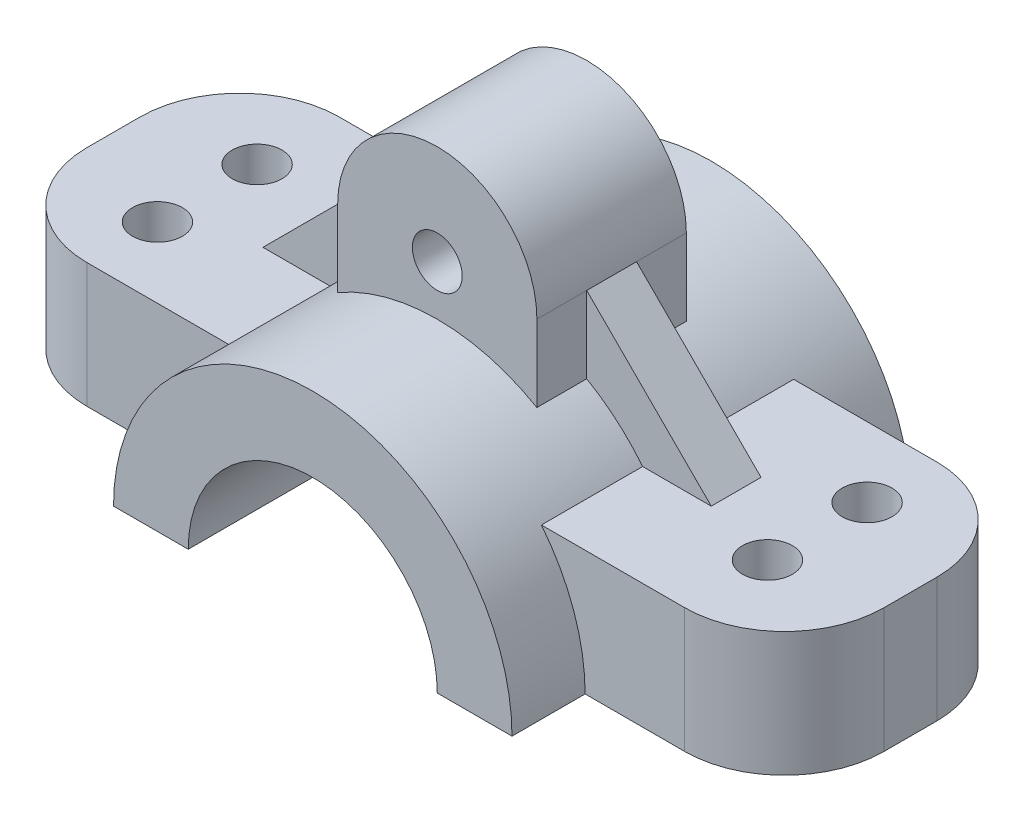
ISO-10303-21;
HEADER;
FILE_DESCRIPTION(('STEP AP214'),'2;1');
FILE_NAME('part.step','',(''),(''),'','','');
FILE_SCHEMA(('AUTOMOTIVE_DESIGN { 1 0 10303 214 1 1 1 1 }'));
ENDSEC;
DATA;
#1=APPLICATION_CONTEXT('core data for automotive mechanical design processes');
#2=APPLICATION_PROTOCOL_DEFINITION('international standard','automotive_design',2000,#1);
#3=PRODUCT_CONTEXT('',#1,'mechanical');
#4=PRODUCT('Part','Part','',(#3));
#5=PRODUCT_RELATED_PRODUCT_CATEGORY('part','',(#4));
#6=PRODUCT_DEFINITION_FORMATION('','',#4);
#7=PRODUCT_DEFINITION_CONTEXT('part definition',#1,'design');
#8=PRODUCT_DEFINITION('design','',#6,#7);
#9=PRODUCT_DEFINITION_SHAPE('','',#8);
#10=(LENGTH_UNIT() NAMED_UNIT(*) SI_UNIT(.MILLI.,.METRE.));
#11=(NAMED_UNIT(*) PLANE_ANGLE_UNIT() SI_UNIT($,.RADIAN.));
#12=(NAMED_UNIT(*) SI_UNIT($,.STERADIAN.) SOLID_ANGLE_UNIT());
#13=UNCERTAINTY_MEASURE_WITH_UNIT(LENGTH_MEASURE(1.E-05),#10,'distance_accuracy_value','');
#14=(GEOMETRIC_REPRESENTATION_CONTEXT(3) GLOBAL_UNCERTAINTY_ASSIGNED_CONTEXT((#13)) GLOBAL_UNIT_ASSIGNED_CONTEXT((#10,
#11,#12)) REPRESENTATION_CONTEXT('',''));
#15=CARTESIAN_POINT('',(0.,0.,0.));
#16=DIRECTION('',(0.,0.,1.));
#17=DIRECTION('',(1.,0.,0.));
#18=AXIS2_PLACEMENT_3D('',#15,#16,#17);
#19=CARTESIAN_POINT('',(0.,0.,-40.));
#20=DIRECTION('',(0.,0.,1.));
#21=DIRECTION('',(1.,0.,0.));
#22=AXIS2_PLACEMENT_3D('',#19,#20,#21);
#23=CYLINDRICAL_SURFACE('',#22,40.);
#24=DIRECTION('',(0.,0.,-1.));
#25=VECTOR('',#24,1.);
#26=CARTESIAN_POINT('',(20.,34.6410161513775,15.));
#27=LINE('',#26,#25);
#28=CARTESIAN_POINT('',(20.,34.6410161513775,-5.));
#29=VERTEX_POINT('',#28);
#30=CARTESIAN_POINT('',(20.,34.6410161513775,-15.));
#31=VERTEX_POINT('',#30);
#32=EDGE_CURVE('E248',#29,#31,#27,.T.);
#33=ORIENTED_EDGE('',*,*,#32,.F.);
#34=CARTESIAN_POINT('',(0.,0.,-5.));
#35=DIRECTION('',(0.,0.,1.));
#36=DIRECTION('',(1.,0.,0.));
#37=AXIS2_PLACEMENT_3D('',#34,#35,#36);
#38=CIRCLE('',#37,40.);
#39=CARTESIAN_POINT('',(31.224989991992,25.,-5.));
#40=VERTEX_POINT('',#39);
#41=EDGE_CURVE('E250',#29,#40,#38,.F.);
#42=ORIENTED_EDGE('',*,*,#41,.T.);
#43=DIRECTION('',(0.,0.,1.));
#44=VECTOR('',#43,1.);
#45=CARTESIAN_POINT('',(31.224989991992,25.,-40.));
#46=LINE('',#45,#44);
#47=CARTESIAN_POINT('',(31.224989991992,25.,-25.3211824849969));
#48=VERTEX_POINT('',#47);
#49=EDGE_CURVE('E229',#40,#48,#46,.F.);
#50=ORIENTED_EDGE('',*,*,#49,.T.);
#51=CARTESIAN_POINT('',(0.,0.,-25.3211824849969));
#52=DIRECTION('',(0.,0.,1.));
#53=DIRECTION('',(1.,0.,0.));
#54=AXIS2_PLACEMENT_3D('',#51,#52,#53);
#55=CIRCLE('',#54,40.);
#56=CARTESIAN_POINT('',(40.,0.,-25.3211824849969));
#57=VERTEX_POINT('',#56);
#58=EDGE_CURVE('E351',#48,#57,#55,.F.);
#59=ORIENTED_EDGE('',*,*,#58,.T.);
#60=DIRECTION('',(0.,0.,1.));
#61=VECTOR('',#60,1.);
#62=CARTESIAN_POINT('',(40.,0.,-40.));
#63=LINE('',#62,#61);
#64=CARTESIAN_POINT('',(40.,0.,-40.));
#65=VERTEX_POINT('',#64);
#66=EDGE_CURVE('E408',#65,#57,#63,.T.);
#67=ORIENTED_EDGE('',*,*,#66,.F.);
#68=CARTESIAN_POINT('',(0.,0.,-40.));
#69=DIRECTION('',(0.,0.,1.));
#70=DIRECTION('',(1.,0.,0.));
#71=AXIS2_PLACEMENT_3D('',#68,#69,#70);
#72=CIRCLE('',#71,40.);
#73=CARTESIAN_POINT('',(-40.,0.,-40.));
#74=VERTEX_POINT('',#73);
#75=EDGE_CURVE('E386',#65,#74,#72,.T.);
#76=ORIENTED_EDGE('',*,*,#75,.T.);
#77=DIRECTION('',(0.,0.,1.));
#78=VECTOR('',#77,1.);
#79=CARTESIAN_POINT('',(-40.,0.,-40.));
#80=LINE('',#79,#78);
#81=CARTESIAN_POINT('',(-40.,0.,-25.3211824849969));
#82=VERTEX_POINT('',#81);
#83=EDGE_CURVE('E416',#74,#82,#80,.T.);
#84=ORIENTED_EDGE('',*,*,#83,.T.);
#85=CARTESIAN_POINT('',(0.,0.,-25.3211824849969));
#86=DIRECTION('',(0.,0.,1.));
#87=DIRECTION('',(1.,0.,0.));
#88=AXIS2_PLACEMENT_3D('',#85,#86,#87);
#89=CIRCLE('',#88,40.);
#90=CARTESIAN_POINT('',(-31.224989991992,25.,-25.3211824849969));
#91=VERTEX_POINT('',#90);
#92=EDGE_CURVE('E346',#82,#91,#89,.F.);
#93=ORIENTED_EDGE('',*,*,#92,.T.);
#94=DIRECTION('',(0.,0.,1.));
#95=VECTOR('',#94,1.);
#96=CARTESIAN_POINT('',(-31.224989991992,25.,-40.));
#97=LINE('',#96,#95);
#98=CARTESIAN_POINT('',(-31.224989991992,25.,-5.));
#99=VERTEX_POINT('',#98);
#100=EDGE_CURVE('E243',#91,#99,#97,.T.);
#101=ORIENTED_EDGE('',*,*,#100,.T.);
#102=CARTESIAN_POINT('',(0.,0.,-5.));
#103=DIRECTION('',(0.,0.,1.));
#104=DIRECTION('',(1.,0.,0.));
#105=AXIS2_PLACEMENT_3D('',#102,#103,#104);
#106=CIRCLE('',#105,40.);
#107=CARTESIAN_POINT('',(-20.,34.6410161513775,-5.));
#108=VERTEX_POINT('',#107);
#109=EDGE_CURVE('E285',#99,#108,#106,.F.);
#110=ORIENTED_EDGE('',*,*,#109,.T.);
#111=DIRECTION('',(0.,0.,1.));
#112=VECTOR('',#111,1.);
#113=CARTESIAN_POINT('',(-20.,34.6410161513775,-40.));
#114=LINE('',#113,#112);
#115=CARTESIAN_POINT('',(-20.,34.6410161513775,-15.));
#116=VERTEX_POINT('',#115);
#117=EDGE_CURVE('E425',#108,#116,#114,.F.);
#118=ORIENTED_EDGE('',*,*,#117,.T.);
#119=CARTESIAN_POINT('',(0.,0.,-15.));
#120=DIRECTION('',(0.,0.,1.));
#121=DIRECTION('',(1.,0.,0.));
#122=AXIS2_PLACEMENT_3D('',#119,#120,#121);
#123=CIRCLE('',#122,40.);
#124=EDGE_CURVE('E415',#116,#31,#123,.F.);
#125=ORIENTED_EDGE('',*,*,#124,.T.);
#126=EDGE_LOOP('',(#33,#42,#50,#59,#67,#76,#84,#93,#101,#110,#118,#125));
#127=FACE_BOUND('',#126,.T.);
#128=ADVANCED_FACE('F44',(#127),#23,.T.);
#129=CARTESIAN_POINT('',(20.,50.,15.));
#130=DIRECTION('',(-1.,0.,0.));
#131=DIRECTION('',(0.,0.,1.));
#132=AXIS2_PLACEMENT_3D('',#129,#130,#131);
#133=PLANE('',#132);
#134=DIRECTION('',(0.,1.,0.));
#135=VECTOR('',#134,1.);
#136=CARTESIAN_POINT('',(20.,50.,-5.));
#137=LINE('',#136,#135);
#138=CARTESIAN_POINT('',(20.,50.,-5.));
#139=VERTEX_POINT('',#138);
#140=EDGE_CURVE('E255',#29,#139,#137,.T.);
#141=ORIENTED_EDGE('',*,*,#140,.F.);
#142=ORIENTED_EDGE('',*,*,#32,.T.);
#143=DIRECTION('',(0.,1.,0.));
#144=VECTOR('',#143,1.);
#145=CARTESIAN_POINT('',(20.,50.,-15.));
#146=LINE('',#145,#144);
#147=CARTESIAN_POINT('',(20.,50.,-15.));
#148=VERTEX_POINT('',#147);
#149=EDGE_CURVE('E366',#31,#148,#146,.T.);
#150=ORIENTED_EDGE('',*,*,#149,.T.);
#151=DIRECTION('',(0.,0.,-1.));
#152=VECTOR('',#151,1.);
#153=CARTESIAN_POINT('',(20.,50.,15.));
#154=LINE('',#153,#152);
#155=EDGE_CURVE('E58',#139,#148,#154,.T.);
#156=ORIENTED_EDGE('',*,*,#155,.F.);
#157=EDGE_LOOP('',(#141,#142,#150,#156));
#158=FACE_BOUND('',#157,.T.);
#159=ADVANCED_FACE('F529',(#158),#133,.F.);
#160=CARTESIAN_POINT('',(-20.,50.,15.));
#161=DIRECTION('',(1.,0.,0.));
#162=DIRECTION('',(0.,0.,-1.));
#163=AXIS2_PLACEMENT_3D('',#160,#161,#162);
#164=PLANE('',#163);
#165=DIRECTION('',(0.,-1.,0.));
#166=VECTOR('',#165,1.);
#167=CARTESIAN_POINT('',(-20.,50.,-5.));
#168=LINE('',#167,#166);
#169=CARTESIAN_POINT('',(-20.,50.,-5.));
#170=VERTEX_POINT('',#169);
#171=EDGE_CURVE('E284',#170,#108,#168,.T.);
#172=ORIENTED_EDGE('',*,*,#171,.F.);
#173=DIRECTION('',(0.,0.,-1.));
#174=VECTOR('',#173,1.);
#175=CARTESIAN_POINT('',(-20.,50.,15.));
#176=LINE('',#175,#174);
#177=CARTESIAN_POINT('',(-20.,50.,-15.));
#178=VERTEX_POINT('',#177);
#179=EDGE_CURVE('E382',#170,#178,#176,.T.);
#180=ORIENTED_EDGE('',*,*,#179,.T.);
#181=DIRECTION('',(0.,-1.,0.));
#182=VECTOR('',#181,1.);
#183=CARTESIAN_POINT('',(-20.,50.,-15.));
#184=LINE('',#183,#182);
#185=EDGE_CURVE('E373',#178,#116,#184,.T.);
#186=ORIENTED_EDGE('',*,*,#185,.T.);
#187=ORIENTED_EDGE('',*,*,#117,.F.);
#188=EDGE_LOOP('',(#172,#180,#186,#187));
#189=FACE_BOUND('',#188,.T.);
#190=ADVANCED_FACE('F518',(#189),#164,.F.);
#191=CARTESIAN_POINT('',(0.,0.,5.));
#192=DIRECTION('',(0.,0.,1.));
#193=DIRECTION('',(1.,0.,0.));
#194=AXIS2_PLACEMENT_3D('',#191,#192,#193);
#195=CIRCLE('',#194,40.);
#196=CARTESIAN_POINT('',(20.,34.6410161513775,5.));
#197=VERTEX_POINT('',#196);
#198=CARTESIAN_POINT('',(31.224989991992,25.,5.));
#199=VERTEX_POINT('',#198);
#200=EDGE_CURVE('E258',#197,#199,#195,.F.);
#201=ORIENTED_EDGE('',*,*,#200,.F.);
#202=CARTESIAN_POINT('',(20.,34.6410161513775,15.));
#203=VERTEX_POINT('',#202);
#204=EDGE_CURVE('E378',#203,#197,#27,.T.);
#205=ORIENTED_EDGE('',*,*,#204,.F.);
#206=CARTESIAN_POINT('',(0.,0.,15.));
#207=DIRECTION('',(0.,0.,1.));
#208=DIRECTION('',(1.,0.,0.));
#209=AXIS2_PLACEMENT_3D('',#206,#207,#208);
#210=CIRCLE('',#209,40.);
#211=CARTESIAN_POINT('',(-20.,34.6410161513775,15.));
#212=VERTEX_POINT('',#211);
#213=EDGE_CURVE('E423',#212,#203,#210,.F.);
#214=ORIENTED_EDGE('',*,*,#213,.F.);
#215=CARTESIAN_POINT('',(-20.,34.6410161513775,5.));
#216=VERTEX_POINT('',#215);
#217=EDGE_CURVE('E424',#212,#216,#114,.F.);
#218=ORIENTED_EDGE('',*,*,#217,.T.);
#219=CARTESIAN_POINT('',(0.,0.,5.));
#220=DIRECTION('',(0.,0.,1.));
#221=DIRECTION('',(1.,0.,0.));
#222=AXIS2_PLACEMENT_3D('',#219,#220,#221);
#223=CIRCLE('',#222,40.);
#224=CARTESIAN_POINT('',(-31.224989991992,25.,5.));
#225=VERTEX_POINT('',#224);
#226=EDGE_CURVE('E273',#225,#216,#223,.F.);
#227=ORIENTED_EDGE('',*,*,#226,.F.);
#228=CARTESIAN_POINT('',(-31.224989991992,25.,25.3211824849969));
#229=VERTEX_POINT('',#228);
#230=EDGE_CURVE('E426',#225,#229,#97,.T.);
#231=ORIENTED_EDGE('',*,*,#230,.T.);
#232=CARTESIAN_POINT('',(0.,0.,25.3211824849969));
#233=DIRECTION('',(0.,0.,-1.));
#234=DIRECTION('',(-1.,0.,0.));
#235=AXIS2_PLACEMENT_3D('',#232,#233,#234);
#236=CIRCLE('',#235,40.);
#237=CARTESIAN_POINT('',(-40.,0.,25.3211824849969));
#238=VERTEX_POINT('',#237);
#239=EDGE_CURVE('E324',#229,#238,#236,.F.);
#240=ORIENTED_EDGE('',*,*,#239,.T.);
#241=CARTESIAN_POINT('',(-40.,0.,40.));
#242=VERTEX_POINT('',#241);
#243=EDGE_CURVE('E396',#238,#242,#80,.T.);
#244=ORIENTED_EDGE('',*,*,#243,.T.);
#245=CARTESIAN_POINT('',(0.,0.,40.));
#246=DIRECTION('',(0.,0.,1.));
#247=DIRECTION('',(1.,0.,0.));
#248=AXIS2_PLACEMENT_3D('',#245,#246,#247);
#249=CIRCLE('',#248,40.);
#250=CARTESIAN_POINT('',(40.,0.,40.));
#251=VERTEX_POINT('',#250);
#252=EDGE_CURVE('E383',#251,#242,#249,.T.);
#253=ORIENTED_EDGE('',*,*,#252,.F.);
#254=CARTESIAN_POINT('',(40.,0.,25.3211824849969));
#255=VERTEX_POINT('',#254);
#256=EDGE_CURVE('E411',#255,#251,#63,.T.);
#257=ORIENTED_EDGE('',*,*,#256,.F.);
#258=CARTESIAN_POINT('',(0.,0.,25.3211824849969));
#259=DIRECTION('',(0.,0.,-1.));
#260=DIRECTION('',(-1.,0.,0.));
#261=AXIS2_PLACEMENT_3D('',#258,#259,#260);
#262=CIRCLE('',#261,40.);
#263=CARTESIAN_POINT('',(31.224989991992,25.,25.3211824849969));
#264=VERTEX_POINT('',#263);
#265=EDGE_CURVE('E347',#255,#264,#262,.F.);
#266=ORIENTED_EDGE('',*,*,#265,.T.);
#267=EDGE_CURVE('E245',#264,#199,#46,.F.);
#268=ORIENTED_EDGE('',*,*,#267,.T.);
#269=EDGE_LOOP('',(#201,#205,#214,#218,#227,#231,#240,#244,#253,#257,#266,#268));
#270=FACE_BOUND('',#269,.T.);
#271=ADVANCED_FACE('F499',(#270),#23,.T.);
#272=CARTESIAN_POINT('',(0.,0.,-40.));
#273=DIRECTION('',(0.,0.,1.));
#274=DIRECTION('',(1.,0.,0.));
#275=AXIS2_PLACEMENT_3D('',#272,#273,#274);
#276=CYLINDRICAL_SURFACE('',#275,25.);
#277=CARTESIAN_POINT('',(0.,0.,40.));
#278=DIRECTION('',(0.,0.,-1.));
#279=DIRECTION('',(1.,0.,0.));
#280=AXIS2_PLACEMENT_3D('',#277,#278,#279);
#281=CIRCLE('',#280,25.);
#282=CARTESIAN_POINT('',(-25.,0.,40.));
#283=VERTEX_POINT('',#282);
#284=CARTESIAN_POINT('',(25.,0.,40.));
#285=VERTEX_POINT('',#284);
#286=EDGE_CURVE('E404',#283,#285,#281,.T.);
#287=ORIENTED_EDGE('',*,*,#286,.F.);
#288=DIRECTION('',(0.,0.,1.));
#289=VECTOR('',#288,1.);
#290=CARTESIAN_POINT('',(-25.,0.,-40.));
#291=LINE('',#290,#289);
#292=CARTESIAN_POINT('',(-25.,0.,-40.));
#293=VERTEX_POINT('',#292);
#294=EDGE_CURVE('E418',#293,#283,#291,.T.);
#295=ORIENTED_EDGE('',*,*,#294,.F.);
#296=CARTESIAN_POINT('',(0.,0.,-40.));
#297=DIRECTION('',(0.,0.,-1.));
#298=DIRECTION('',(1.,0.,0.));
#299=AXIS2_PLACEMENT_3D('',#296,#297,#298);
#300=CIRCLE('',#299,25.);
#301=CARTESIAN_POINT('',(25.,0.,-40.));
#302=VERTEX_POINT('',#301);
#303=EDGE_CURVE('E391',#293,#302,#300,.T.);
#304=ORIENTED_EDGE('',*,*,#303,.T.);
#305=DIRECTION('',(0.,0.,1.));
#306=VECTOR('',#305,1.);
#307=CARTESIAN_POINT('',(25.,0.,-40.));
#308=LINE('',#307,#306);
#309=EDGE_CURVE('E414',#302,#285,#308,.T.);
#310=ORIENTED_EDGE('',*,*,#309,.T.);
#311=EDGE_LOOP('',(#287,#295,#304,#310));
#312=FACE_BOUND('',#311,.T.);
#313=ADVANCED_FACE('F575',(#312),#276,.F.);
#314=CARTESIAN_POINT('',(25.,0.,-40.));
#315=DIRECTION('',(0.,-1.,0.));
#316=DIRECTION('',(0.,0.,-1.));
#317=AXIS2_PLACEMENT_3D('',#314,#315,#316);
#318=PLANE('',#317);
#319=CARTESIAN_POINT('',(60.,0.,8.71133105624287));
#320=DIRECTION('',(0.,1.,0.));
#321=DIRECTION('',(0.,0.,1.));
#322=AXIS2_PLACEMENT_3D('',#319,#320,#321);
#323=CIRCLE('',#322,5.);
#324=CARTESIAN_POINT('',(60.,0.,13.7113310562429));
#325=VERTEX_POINT('',#324);
#326=EDGE_CURVE('E291',#325,#325,#323,.T.);
#327=ORIENTED_EDGE('',*,*,#326,.T.);
#328=EDGE_LOOP('',(#327));
#329=FACE_BOUND('',#328,.T.);
#330=DIRECTION('',(1.,0.,0.));
#331=VECTOR('',#330,1.);
#332=CARTESIAN_POINT('',(25.,0.,40.));
#333=LINE('',#332,#331);
#334=EDGE_CURVE('E389',#285,#251,#333,.T.);
#335=ORIENTED_EDGE('',*,*,#334,.F.);
#336=ORIENTED_EDGE('',*,*,#309,.F.);
#337=DIRECTION('',(1.,0.,0.));
#338=VECTOR('',#337,1.);
#339=CARTESIAN_POINT('',(25.,0.,-40.));
#340=LINE('',#339,#338);
#341=EDGE_CURVE('E392',#302,#65,#340,.T.);
#342=ORIENTED_EDGE('',*,*,#341,.T.);
#343=ORIENTED_EDGE('',*,*,#66,.T.);
#344=DIRECTION('',(-1.,0.,0.));
#345=VECTOR('',#344,1.);
#346=CARTESIAN_POINT('',(10.,0.,-25.3211824849969));
#347=LINE('',#346,#345);
#348=CARTESIAN_POINT('',(60.,0.,-25.3211824849969));
#349=VERTEX_POINT('',#348);
#350=EDGE_CURVE('E328',#349,#57,#347,.T.);
#351=ORIENTED_EDGE('',*,*,#350,.F.);
#352=CARTESIAN_POINT('',(60.,0.,-5.32118248499691));
#353=DIRECTION('',(0.,-1.,0.));
#354=DIRECTION('',(0.,0.,-1.));
#355=AXIS2_PLACEMENT_3D('',#352,#353,#354);
#356=CIRCLE('',#355,20.);
#357=CARTESIAN_POINT('',(80.,0.,-5.32118248499691));
#358=VERTEX_POINT('',#357);
#359=EDGE_CURVE('E440',#349,#358,#356,.T.);
#360=ORIENTED_EDGE('',*,*,#359,.T.);
#361=DIRECTION('',(0.,0.,-1.));
#362=VECTOR('',#361,1.);
#363=CARTESIAN_POINT('',(80.,0.,-25.3211824849969));
#364=LINE('',#363,#362);
#365=CARTESIAN_POINT('',(80.,0.,5.32118248499693));
#366=VERTEX_POINT('',#365);
#367=EDGE_CURVE('E318',#366,#358,#364,.T.);
#368=ORIENTED_EDGE('',*,*,#367,.F.);
#369=CARTESIAN_POINT('',(60.,0.,5.32118248499693));
#370=DIRECTION('',(0.,-1.,0.));
#371=DIRECTION('',(0.,0.,-1.));
#372=AXIS2_PLACEMENT_3D('',#369,#370,#371);
#373=CIRCLE('',#372,20.);
#374=CARTESIAN_POINT('',(60.,0.,25.3211824849969));
#375=VERTEX_POINT('',#374);
#376=EDGE_CURVE('E434',#366,#375,#373,.T.);
#377=ORIENTED_EDGE('',*,*,#376,.T.);
#378=DIRECTION('',(1.,0.,0.));
#379=VECTOR('',#378,1.);
#380=CARTESIAN_POINT('',(9.99999999999999,0.,25.3211824849969));
#381=LINE('',#380,#379);
#382=EDGE_CURVE('E326',#255,#375,#381,.T.);
#383=ORIENTED_EDGE('',*,*,#382,.F.);
#384=ORIENTED_EDGE('',*,*,#256,.T.);
#385=EDGE_LOOP('',(#335,#336,#342,#343,#351,#360,#368,#377,#383,#384));
#386=FACE_BOUND('',#385,.T.);
#387=CARTESIAN_POINT('',(60.,0.,-11.2886689437571));
#388=DIRECTION('',(0.,1.,0.));
#389=DIRECTION('',(0.,0.,1.));
#390=AXIS2_PLACEMENT_3D('',#387,#388,#389);
#391=CIRCLE('',#390,5.);
#392=CARTESIAN_POINT('',(60.,0.,-6.28866894375712));
#393=VERTEX_POINT('',#392);
#394=EDGE_CURVE('E295',#393,#393,#391,.T.);
#395=ORIENTED_EDGE('',*,*,#394,.T.);
#396=EDGE_LOOP('',(#395));
#397=FACE_BOUND('',#396,.T.);
#398=ADVANCED_FACE('F577',(#329,#386,#397),#318,.T.);
#399=CARTESIAN_POINT('',(-40.,0.,-40.));
#400=DIRECTION('',(0.,-1.,0.));
#401=DIRECTION('',(0.,0.,-1.));
#402=AXIS2_PLACEMENT_3D('',#399,#400,#401);
#403=PLANE('',#402);
#404=CARTESIAN_POINT('',(-60.,0.,5.32118248499693));
#405=DIRECTION('',(0.,-1.,0.));
#406=DIRECTION('',(0.,0.,-1.));
#407=AXIS2_PLACEMENT_3D('',#404,#405,#406);
#408=CIRCLE('',#407,20.);
#409=CARTESIAN_POINT('',(-60.,0.,25.3211824849969));
#410=VERTEX_POINT('',#409);
#411=CARTESIAN_POINT('',(-80.,0.,5.32118248499693));
#412=VERTEX_POINT('',#411);
#413=EDGE_CURVE('E454',#410,#412,#408,.T.);
#414=ORIENTED_EDGE('',*,*,#413,.T.);
#415=DIRECTION('',(0.,0.,1.));
#416=VECTOR('',#415,1.);
#417=CARTESIAN_POINT('',(-80.,0.,-25.3211824849969));
#418=LINE('',#417,#416);
#419=CARTESIAN_POINT('',(-80.,0.,-5.32118248499691));
#420=VERTEX_POINT('',#419);
#421=EDGE_CURVE('E334',#420,#412,#418,.T.);
#422=ORIENTED_EDGE('',*,*,#421,.F.);
#423=CARTESIAN_POINT('',(-60.,0.,-5.32118248499691));
#424=DIRECTION('',(0.,-1.,0.));
#425=DIRECTION('',(0.,0.,-1.));
#426=AXIS2_PLACEMENT_3D('',#423,#424,#425);
#427=CIRCLE('',#426,20.);
#428=CARTESIAN_POINT('',(-60.,0.,-25.3211824849969));
#429=VERTEX_POINT('',#428);
#430=EDGE_CURVE('E467',#420,#429,#427,.T.);
#431=ORIENTED_EDGE('',*,*,#430,.T.);
#432=DIRECTION('',(-1.,0.,0.));
#433=VECTOR('',#432,1.);
#434=CARTESIAN_POINT('',(-10.,0.,-25.3211824849969));
#435=LINE('',#434,#433);
#436=EDGE_CURVE('E329',#82,#429,#435,.T.);
#437=ORIENTED_EDGE('',*,*,#436,.F.);
#438=ORIENTED_EDGE('',*,*,#83,.F.);
#439=DIRECTION('',(1.,0.,0.));
#440=VECTOR('',#439,1.);
#441=CARTESIAN_POINT('',(-40.,0.,-40.));
#442=LINE('',#441,#440);
#443=EDGE_CURVE('E388',#74,#293,#442,.T.);
#444=ORIENTED_EDGE('',*,*,#443,.T.);
#445=ORIENTED_EDGE('',*,*,#294,.T.);
#446=DIRECTION('',(1.,0.,0.));
#447=VECTOR('',#446,1.);
#448=CARTESIAN_POINT('',(-40.,0.,40.));
#449=LINE('',#448,#447);
#450=EDGE_CURVE('E402',#242,#283,#449,.T.);
#451=ORIENTED_EDGE('',*,*,#450,.F.);
#452=ORIENTED_EDGE('',*,*,#243,.F.);
#453=DIRECTION('',(1.,0.,0.));
#454=VECTOR('',#453,1.);
#455=CARTESIAN_POINT('',(-9.99999999999999,0.,25.3211824849969));
#456=LINE('',#455,#454);
#457=EDGE_CURVE('E331',#410,#238,#456,.T.);
#458=ORIENTED_EDGE('',*,*,#457,.F.);
#459=EDGE_LOOP('',(#414,#422,#431,#437,#438,#444,#445,#451,#452,#458));
#460=FACE_BOUND('',#459,.T.);
#461=CARTESIAN_POINT('',(-60.,0.,11.1755474280481));
#462=DIRECTION('',(0.,1.,0.));
#463=DIRECTION('',(0.,0.,1.));
#464=AXIS2_PLACEMENT_3D('',#461,#462,#463);
#465=CIRCLE('',#464,5.);
#466=CARTESIAN_POINT('',(-60.,0.,16.1755474280481));
#467=VERTEX_POINT('',#466);
#468=EDGE_CURVE('E300',#467,#467,#465,.T.);
#469=ORIENTED_EDGE('',*,*,#468,.T.);
#470=EDGE_LOOP('',(#469));
#471=FACE_BOUND('',#470,.T.);
#472=CARTESIAN_POINT('',(-60.,0.,-8.82445257195192));
#473=DIRECTION('',(0.,1.,0.));
#474=DIRECTION('',(0.,0.,1.));
#475=AXIS2_PLACEMENT_3D('',#472,#473,#474);
#476=CIRCLE('',#475,5.);
#477=CARTESIAN_POINT('',(-60.,0.,-3.82445257195192));
#478=VERTEX_POINT('',#477);
#479=EDGE_CURVE('E306',#478,#478,#476,.T.);
#480=ORIENTED_EDGE('',*,*,#479,.T.);
#481=EDGE_LOOP('',(#480));
#482=FACE_BOUND('',#481,.T.);
#483=ADVANCED_FACE('F484',(#460,#471,#482),#403,.T.);
#484=CARTESIAN_POINT('',(0.,0.,-40.));
#485=DIRECTION('',(0.,0.,1.));
#486=DIRECTION('',(1.,0.,0.));
#487=AXIS2_PLACEMENT_3D('',#484,#485,#486);
#488=PLANE('',#487);
#489=ORIENTED_EDGE('',*,*,#75,.F.);
#490=ORIENTED_EDGE('',*,*,#341,.F.);
#491=ORIENTED_EDGE('',*,*,#303,.F.);
#492=ORIENTED_EDGE('',*,*,#443,.F.);
#493=EDGE_LOOP('',(#489,#490,#491,#492));
#494=FACE_BOUND('',#493,.T.);
#495=ADVANCED_FACE('F590',(#494),#488,.F.);
#496=CARTESIAN_POINT('',(0.,0.,40.));
#497=DIRECTION('',(0.,0.,1.));
#498=DIRECTION('',(1.,0.,0.));
#499=AXIS2_PLACEMENT_3D('',#496,#497,#498);
#500=PLANE('',#499);
#501=ORIENTED_EDGE('',*,*,#252,.T.);
#502=ORIENTED_EDGE('',*,*,#450,.T.);
#503=ORIENTED_EDGE('',*,*,#286,.T.);
#504=ORIENTED_EDGE('',*,*,#334,.T.);
#505=EDGE_LOOP('',(#501,#502,#503,#504));
#506=FACE_BOUND('',#505,.T.);
#507=ADVANCED_FACE('F593',(#506),#500,.T.);
#508=CARTESIAN_POINT('',(0.,50.,15.));
#509=DIRECTION('',(0.,0.,1.));
#510=DIRECTION('',(1.,0.,0.));
#511=AXIS2_PLACEMENT_3D('',#508,#509,#510);
#512=PLANE('',#511);
#513=DIRECTION('',(0.,-1.,0.));
#514=VECTOR('',#513,1.);
#515=CARTESIAN_POINT('',(-20.,50.,15.));
#516=LINE('',#515,#514);
#517=CARTESIAN_POINT('',(-20.,50.,15.));
#518=VERTEX_POINT('',#517);
#519=EDGE_CURVE('E362',#518,#212,#516,.T.);
#520=ORIENTED_EDGE('',*,*,#519,.T.);
#521=ORIENTED_EDGE('',*,*,#213,.T.);
#522=DIRECTION('',(0.,1.,0.));
#523=VECTOR('',#522,1.);
#524=CARTESIAN_POINT('',(20.,50.,15.));
#525=LINE('',#524,#523);
#526=CARTESIAN_POINT('',(20.,50.,15.));
#527=VERTEX_POINT('',#526);
#528=EDGE_CURVE('E367',#203,#527,#525,.T.);
#529=ORIENTED_EDGE('',*,*,#528,.T.);
#530=CARTESIAN_POINT('',(0.,50.,15.));
#531=DIRECTION('',(0.,0.,1.));
#532=DIRECTION('',(1.,0.,0.));
#533=AXIS2_PLACEMENT_3D('',#530,#531,#532);
#534=CIRCLE('',#533,20.);
#535=EDGE_CURVE('E365',#527,#518,#534,.T.);
#536=ORIENTED_EDGE('',*,*,#535,.T.);
#537=EDGE_LOOP('',(#520,#521,#529,#536));
#538=FACE_BOUND('',#537,.T.);
#539=CARTESIAN_POINT('',(0.,50.,15.));
#540=DIRECTION('',(0.,0.,1.));
#541=DIRECTION('',(1.,0.,0.));
#542=AXIS2_PLACEMENT_3D('',#539,#540,#541);
#543=CIRCLE('',#542,5.);
#544=CARTESIAN_POINT('',(5.,50.,15.));
#545=VERTEX_POINT('',#544);
#546=EDGE_CURVE('E358',#545,#545,#543,.T.);
#547=ORIENTED_EDGE('',*,*,#546,.F.);
#548=EDGE_LOOP('',(#547));
#549=FACE_BOUND('',#548,.T.);
#550=ADVANCED_FACE('F547',(#538,#549),#512,.T.);
#551=CARTESIAN_POINT('',(0.,50.,-15.));
#552=DIRECTION('',(0.,0.,1.));
#553=DIRECTION('',(1.,0.,0.));
#554=AXIS2_PLACEMENT_3D('',#551,#552,#553);
#555=PLANE('',#554);
#556=ORIENTED_EDGE('',*,*,#124,.F.);
#557=ORIENTED_EDGE('',*,*,#185,.F.);
#558=CARTESIAN_POINT('',(0.,50.,-15.));
#559=DIRECTION('',(0.,0.,1.));
#560=DIRECTION('',(1.,0.,0.));
#561=AXIS2_PLACEMENT_3D('',#558,#559,#560);
#562=CIRCLE('',#561,20.);
#563=EDGE_CURVE('E360',#148,#178,#562,.T.);
#564=ORIENTED_EDGE('',*,*,#563,.F.);
#565=ORIENTED_EDGE('',*,*,#149,.F.);
#566=EDGE_LOOP('',(#556,#557,#564,#565));
#567=FACE_BOUND('',#566,.T.);
#568=CARTESIAN_POINT('',(0.,50.,-15.));
#569=DIRECTION('',(0.,0.,1.));
#570=DIRECTION('',(1.,0.,0.));
#571=AXIS2_PLACEMENT_3D('',#568,#569,#570);
#572=CIRCLE('',#571,5.);
#573=CARTESIAN_POINT('',(5.,50.,-15.));
#574=VERTEX_POINT('',#573);
#575=EDGE_CURVE('E354',#574,#574,#572,.T.);
#576=ORIENTED_EDGE('',*,*,#575,.T.);
#577=EDGE_LOOP('',(#576));
#578=FACE_BOUND('',#577,.T.);
#579=ADVANCED_FACE('F524',(#567,#578),#555,.F.);
#580=CARTESIAN_POINT('',(0.,50.,15.));
#581=DIRECTION('',(0.,0.,-1.));
#582=DIRECTION('',(-1.,0.,0.));
#583=AXIS2_PLACEMENT_3D('',#580,#581,#582);
#584=CYLINDRICAL_SURFACE('',#583,20.);
#585=DIRECTION('',(0.,0.,1.));
#586=VECTOR('',#585,1.);
#587=CARTESIAN_POINT('',(-20.,49.9999999999999,15.));
#588=LINE('',#587,#586);
#589=CARTESIAN_POINT('',(-20.,50.,5.));
#590=VERTEX_POINT('',#589);
#591=EDGE_CURVE('E293',#170,#590,#588,.T.);
#592=ORIENTED_EDGE('',*,*,#591,.T.);
#593=EDGE_CURVE('E385',#518,#590,#176,.T.);
#594=ORIENTED_EDGE('',*,*,#593,.F.);
#595=ORIENTED_EDGE('',*,*,#535,.F.);
#596=CARTESIAN_POINT('',(20.,50.,5.));
#597=VERTEX_POINT('',#596);
#598=EDGE_CURVE('E380',#527,#597,#154,.T.);
#599=ORIENTED_EDGE('',*,*,#598,.T.);
#600=DIRECTION('',(0.,0.,1.));
#601=VECTOR('',#600,1.);
#602=CARTESIAN_POINT('',(20.,50.,15.));
#603=LINE('',#602,#601);
#604=EDGE_CURVE('E268',#597,#139,#603,.F.);
#605=ORIENTED_EDGE('',*,*,#604,.T.);
#606=ORIENTED_EDGE('',*,*,#155,.T.);
#607=ORIENTED_EDGE('',*,*,#563,.T.);
#608=ORIENTED_EDGE('',*,*,#179,.F.);
#609=EDGE_LOOP('',(#592,#594,#595,#599,#605,#606,#607,#608));
#610=FACE_BOUND('',#609,.T.);
#611=ADVANCED_FACE('F526',(#610),#584,.T.);
#612=ORIENTED_EDGE('',*,*,#593,.T.);
#613=DIRECTION('',(0.,-1.,0.));
#614=VECTOR('',#613,1.);
#615=CARTESIAN_POINT('',(-20.,50.,5.));
#616=LINE('',#615,#614);
#617=EDGE_CURVE('E277',#590,#216,#616,.T.);
#618=ORIENTED_EDGE('',*,*,#617,.T.);
#619=ORIENTED_EDGE('',*,*,#217,.F.);
#620=ORIENTED_EDGE('',*,*,#519,.F.);
#621=EDGE_LOOP('',(#612,#618,#619,#620));
#622=FACE_BOUND('',#621,.T.);
#623=ADVANCED_FACE('F552',(#622),#164,.F.);
#624=ORIENTED_EDGE('',*,*,#204,.T.);
#625=DIRECTION('',(0.,1.,0.));
#626=VECTOR('',#625,1.);
#627=CARTESIAN_POINT('',(20.,50.,5.));
#628=LINE('',#627,#626);
#629=EDGE_CURVE('E66',#197,#597,#628,.T.);
#630=ORIENTED_EDGE('',*,*,#629,.T.);
#631=ORIENTED_EDGE('',*,*,#598,.F.);
#632=ORIENTED_EDGE('',*,*,#528,.F.);
#633=EDGE_LOOP('',(#624,#630,#631,#632));
#634=FACE_BOUND('',#633,.T.);
#635=ADVANCED_FACE('F548',(#634),#133,.F.);
#636=CARTESIAN_POINT('',(0.,50.,15.));
#637=DIRECTION('',(0.,0.,-1.));
#638=DIRECTION('',(-1.,0.,0.));
#639=AXIS2_PLACEMENT_3D('',#636,#637,#638);
#640=CYLINDRICAL_SURFACE('',#639,5.);
#641=ORIENTED_EDGE('',*,*,#546,.T.);
#642=EDGE_LOOP('',(#641));
#643=FACE_BOUND('',#642,.T.);
#644=ORIENTED_EDGE('',*,*,#575,.F.);
#645=EDGE_LOOP('',(#644));
#646=FACE_BOUND('',#645,.T.);
#647=ADVANCED_FACE('F557',(#643,#646),#640,.F.);
#648=CARTESIAN_POINT('',(-10.,25.,-25.3211824849969));
#649=DIRECTION('',(0.,0.,1.));
#650=DIRECTION('',(1.,0.,0.));
#651=AXIS2_PLACEMENT_3D('',#648,#649,#650);
#652=PLANE('',#651);
#653=ORIENTED_EDGE('',*,*,#436,.T.);
#654=DIRECTION('',(0.,-1.,0.));
#655=VECTOR('',#654,1.);
#656=CARTESIAN_POINT('',(-60.,25.,-25.3211824849969));
#657=LINE('',#656,#655);
#658=CARTESIAN_POINT('',(-60.,25.,-25.3211824849969));
#659=VERTEX_POINT('',#658);
#660=EDGE_CURVE('E52',#429,#659,#657,.F.);
#661=ORIENTED_EDGE('',*,*,#660,.T.);
#662=DIRECTION('',(-1.,0.,0.));
#663=VECTOR('',#662,1.);
#664=CARTESIAN_POINT('',(-10.,25.,-25.3211824849969));
#665=LINE('',#664,#663);
#666=EDGE_CURVE('E337',#91,#659,#665,.T.);
#667=ORIENTED_EDGE('',*,*,#666,.F.);
#668=ORIENTED_EDGE('',*,*,#92,.F.);
#669=EDGE_LOOP('',(#653,#661,#667,#668));
#670=FACE_BOUND('',#669,.T.);
#671=ADVANCED_FACE('F468',(#670),#652,.F.);
#672=CARTESIAN_POINT('',(-9.99999999999999,25.,25.3211824849969));
#673=DIRECTION('',(0.,0.,-1.));
#674=DIRECTION('',(-1.,0.,0.));
#675=AXIS2_PLACEMENT_3D('',#672,#673,#674);
#676=PLANE('',#675);
#677=DIRECTION('',(1.,0.,0.));
#678=VECTOR('',#677,1.);
#679=CARTESIAN_POINT('',(-9.99999999999999,25.,25.3211824849969));
#680=LINE('',#679,#678);
#681=CARTESIAN_POINT('',(-60.,25.,25.3211824849969));
#682=VERTEX_POINT('',#681);
#683=EDGE_CURVE('E307',#682,#229,#680,.T.);
#684=ORIENTED_EDGE('',*,*,#683,.F.);
#685=DIRECTION('',(0.,-1.,0.));
#686=VECTOR('',#685,1.);
#687=CARTESIAN_POINT('',(-60.,25.,25.3211824849969));
#688=LINE('',#687,#686);
#689=EDGE_CURVE('E455',#682,#410,#688,.T.);
#690=ORIENTED_EDGE('',*,*,#689,.T.);
#691=ORIENTED_EDGE('',*,*,#457,.T.);
#692=ORIENTED_EDGE('',*,*,#239,.F.);
#693=EDGE_LOOP('',(#684,#690,#691,#692));
#694=FACE_BOUND('',#693,.T.);
#695=ADVANCED_FACE('F498',(#694),#676,.F.);
#696=CARTESIAN_POINT('',(-80.,25.,-25.3211824849969));
#697=DIRECTION('',(1.,0.,0.));
#698=DIRECTION('',(0.,0.,-1.));
#699=AXIS2_PLACEMENT_3D('',#696,#697,#698);
#700=PLANE('',#699);
#701=DIRECTION('',(0.,-1.,0.));
#702=VECTOR('',#701,1.);
#703=CARTESIAN_POINT('',(-80.,25.,5.32118248499693));
#704=LINE('',#703,#702);
#705=CARTESIAN_POINT('',(-80.,25.,5.32118248499693));
#706=VERTEX_POINT('',#705);
#707=EDGE_CURVE('E456',#412,#706,#704,.F.);
#708=ORIENTED_EDGE('',*,*,#707,.T.);
#709=DIRECTION('',(0.,0.,1.));
#710=VECTOR('',#709,1.);
#711=CARTESIAN_POINT('',(-80.,25.,-25.3211824849969));
#712=LINE('',#711,#710);
#713=CARTESIAN_POINT('',(-80.,25.,-5.32118248499691));
#714=VERTEX_POINT('',#713);
#715=EDGE_CURVE('E345',#714,#706,#712,.T.);
#716=ORIENTED_EDGE('',*,*,#715,.F.);
#717=DIRECTION('',(0.,-1.,0.));
#718=VECTOR('',#717,1.);
#719=CARTESIAN_POINT('',(-80.,25.,-5.32118248499691));
#720=LINE('',#719,#718);
#721=EDGE_CURVE('E461',#714,#420,#720,.T.);
#722=ORIENTED_EDGE('',*,*,#721,.T.);
#723=ORIENTED_EDGE('',*,*,#421,.T.);
#724=EDGE_LOOP('',(#708,#716,#722,#723));
#725=FACE_BOUND('',#724,.T.);
#726=ADVANCED_FACE('F481',(#725),#700,.F.);
#727=CARTESIAN_POINT('',(0.,25.,0.));
#728=DIRECTION('',(0.,-1.,0.));
#729=DIRECTION('',(0.,0.,-1.));
#730=AXIS2_PLACEMENT_3D('',#727,#728,#729);
#731=PLANE('',#730);
#732=DIRECTION('',(-1.,0.,0.));
#733=VECTOR('',#732,1.);
#734=CARTESIAN_POINT('',(0.,25.,5.));
#735=LINE('',#734,#733);
#736=CARTESIAN_POINT('',(-45.,25.,5.));
#737=VERTEX_POINT('',#736);
#738=EDGE_CURVE('E275',#225,#737,#735,.T.);
#739=ORIENTED_EDGE('',*,*,#738,.T.);
#740=DIRECTION('',(0.,0.,-1.));
#741=VECTOR('',#740,1.);
#742=CARTESIAN_POINT('',(-45.,25.,0.));
#743=LINE('',#742,#741);
#744=CARTESIAN_POINT('',(-45.,25.,-5.));
#745=VERTEX_POINT('',#744);
#746=EDGE_CURVE('E287',#737,#745,#743,.T.);
#747=ORIENTED_EDGE('',*,*,#746,.T.);
#748=DIRECTION('',(-1.,0.,0.));
#749=VECTOR('',#748,1.);
#750=CARTESIAN_POINT('',(0.,25.,-5.));
#751=LINE('',#750,#749);
#752=EDGE_CURVE('E283',#99,#745,#751,.T.);
#753=ORIENTED_EDGE('',*,*,#752,.F.);
#754=ORIENTED_EDGE('',*,*,#100,.F.);
#755=ORIENTED_EDGE('',*,*,#666,.T.);
#756=CARTESIAN_POINT('',(-60.,25.,-5.32118248499691));
#757=DIRECTION('',(0.,-1.,0.));
#758=DIRECTION('',(0.,0.,-1.));
#759=AXIS2_PLACEMENT_3D('',#756,#757,#758);
#760=CIRCLE('',#759,20.);
#761=EDGE_CURVE('E11',#659,#714,#760,.F.);
#762=ORIENTED_EDGE('',*,*,#761,.T.);
#763=ORIENTED_EDGE('',*,*,#715,.T.);
#764=CARTESIAN_POINT('',(-60.,25.,5.32118248499693));
#765=DIRECTION('',(0.,-1.,0.));
#766=DIRECTION('',(0.,0.,-1.));
#767=AXIS2_PLACEMENT_3D('',#764,#765,#766);
#768=CIRCLE('',#767,20.);
#769=EDGE_CURVE('E463',#706,#682,#768,.F.);
#770=ORIENTED_EDGE('',*,*,#769,.T.);
#771=ORIENTED_EDGE('',*,*,#683,.T.);
#772=ORIENTED_EDGE('',*,*,#230,.F.);
#773=EDGE_LOOP('',(#739,#747,#753,#754,#755,#762,#763,#770,#771,#772));
#774=FACE_BOUND('',#773,.T.);
#775=CARTESIAN_POINT('',(-60.,25.,11.1755474280481));
#776=DIRECTION('',(0.,1.,0.));
#777=DIRECTION('',(0.,0.,1.));
#778=AXIS2_PLACEMENT_3D('',#775,#776,#777);
#779=CIRCLE('',#778,5.);
#780=CARTESIAN_POINT('',(-60.,25.,16.1755474280481));
#781=VERTEX_POINT('',#780);
#782=EDGE_CURVE('E312',#781,#781,#779,.T.);
#783=ORIENTED_EDGE('',*,*,#782,.F.);
#784=EDGE_LOOP('',(#783));
#785=FACE_BOUND('',#784,.T.);
#786=CARTESIAN_POINT('',(-60.,25.,-8.82445257195192));
#787=DIRECTION('',(0.,1.,0.));
#788=DIRECTION('',(0.,0.,1.));
#789=AXIS2_PLACEMENT_3D('',#786,#787,#788);
#790=CIRCLE('',#789,5.);
#791=CARTESIAN_POINT('',(-60.,25.,-3.82445257195192));
#792=VERTEX_POINT('',#791);
#793=EDGE_CURVE('E309',#792,#792,#790,.T.);
#794=ORIENTED_EDGE('',*,*,#793,.F.);
#795=EDGE_LOOP('',(#794));
#796=FACE_BOUND('',#795,.T.);
#797=ADVANCED_FACE('F480',(#774,#785,#796),#731,.F.);
#798=CARTESIAN_POINT('',(10.,25.,-25.3211824849969));
#799=DIRECTION('',(0.,0.,1.));
#800=DIRECTION('',(1.,0.,0.));
#801=AXIS2_PLACEMENT_3D('',#798,#799,#800);
#802=PLANE('',#801);
#803=DIRECTION('',(-1.,0.,0.));
#804=VECTOR('',#803,1.);
#805=CARTESIAN_POINT('',(10.,25.,-25.3211824849969));
#806=LINE('',#805,#804);
#807=CARTESIAN_POINT('',(60.,25.,-25.3211824849969));
#808=VERTEX_POINT('',#807);
#809=EDGE_CURVE('E238',#808,#48,#806,.T.);
#810=ORIENTED_EDGE('',*,*,#809,.F.);
#811=DIRECTION('',(0.,-1.,0.));
#812=VECTOR('',#811,1.);
#813=CARTESIAN_POINT('',(60.,25.,-25.3211824849969));
#814=LINE('',#813,#812);
#815=EDGE_CURVE('E435',#808,#349,#814,.T.);
#816=ORIENTED_EDGE('',*,*,#815,.T.);
#817=ORIENTED_EDGE('',*,*,#350,.T.);
#818=ORIENTED_EDGE('',*,*,#58,.F.);
#819=EDGE_LOOP('',(#810,#816,#817,#818));
#820=FACE_BOUND('',#819,.T.);
#821=ADVANCED_FACE('F630',(#820),#802,.F.);
#822=CARTESIAN_POINT('',(9.99999999999999,25.,25.3211824849969));
#823=DIRECTION('',(0.,0.,-1.));
#824=DIRECTION('',(-1.,0.,0.));
#825=AXIS2_PLACEMENT_3D('',#822,#823,#824);
#826=PLANE('',#825);
#827=ORIENTED_EDGE('',*,*,#382,.T.);
#828=DIRECTION('',(0.,-1.,0.));
#829=VECTOR('',#828,1.);
#830=CARTESIAN_POINT('',(60.,25.,25.3211824849969));
#831=LINE('',#830,#829);
#832=CARTESIAN_POINT('',(60.,25.,25.3211824849969));
#833=VERTEX_POINT('',#832);
#834=EDGE_CURVE('E448',#375,#833,#831,.F.);
#835=ORIENTED_EDGE('',*,*,#834,.T.);
#836=DIRECTION('',(1.,0.,0.));
#837=VECTOR('',#836,1.);
#838=CARTESIAN_POINT('',(9.99999999999999,25.,25.3211824849969));
#839=LINE('',#838,#837);
#840=EDGE_CURVE('E316',#264,#833,#839,.T.);
#841=ORIENTED_EDGE('',*,*,#840,.F.);
#842=ORIENTED_EDGE('',*,*,#265,.F.);
#843=EDGE_LOOP('',(#827,#835,#841,#842));
#844=FACE_BOUND('',#843,.T.);
#845=ADVANCED_FACE('F611',(#844),#826,.F.);
#846=CARTESIAN_POINT('',(80.,25.,-25.3211824849969));
#847=DIRECTION('',(-1.,0.,0.));
#848=DIRECTION('',(0.,0.,1.));
#849=AXIS2_PLACEMENT_3D('',#846,#847,#848);
#850=PLANE('',#849);
#851=ORIENTED_EDGE('',*,*,#367,.T.);
#852=DIRECTION('',(0.,-1.,0.));
#853=VECTOR('',#852,1.);
#854=CARTESIAN_POINT('',(80.,25.,-5.32118248499691));
#855=LINE('',#854,#853);
#856=CARTESIAN_POINT('',(80.,25.,-5.32118248499691));
#857=VERTEX_POINT('',#856);
#858=EDGE_CURVE('E442',#358,#857,#855,.F.);
#859=ORIENTED_EDGE('',*,*,#858,.T.);
#860=DIRECTION('',(0.,0.,-1.));
#861=VECTOR('',#860,1.);
#862=CARTESIAN_POINT('',(80.,25.,-25.3211824849969));
#863=LINE('',#862,#861);
#864=CARTESIAN_POINT('',(80.,25.,5.32118248499693));
#865=VERTEX_POINT('',#864);
#866=EDGE_CURVE('E322',#865,#857,#863,.T.);
#867=ORIENTED_EDGE('',*,*,#866,.F.);
#868=DIRECTION('',(0.,-1.,0.));
#869=VECTOR('',#868,1.);
#870=CARTESIAN_POINT('',(80.,25.,5.32118248499693));
#871=LINE('',#870,#869);
#872=EDGE_CURVE('E439',#865,#366,#871,.T.);
#873=ORIENTED_EDGE('',*,*,#872,.T.);
#874=EDGE_LOOP('',(#851,#859,#867,#873));
#875=FACE_BOUND('',#874,.T.);
#876=ADVANCED_FACE('F619',(#875),#850,.F.);
#877=CARTESIAN_POINT('',(0.,25.,0.));
#878=DIRECTION('',(0.,-1.,0.));
#879=DIRECTION('',(0.,0.,-1.));
#880=AXIS2_PLACEMENT_3D('',#877,#878,#879);
#881=PLANE('',#880);
#882=CARTESIAN_POINT('',(60.,25.,8.71133105624287));
#883=DIRECTION('',(0.,1.,0.));
#884=DIRECTION('',(0.,0.,1.));
#885=AXIS2_PLACEMENT_3D('',#882,#883,#884);
#886=CIRCLE('',#885,5.);
#887=CARTESIAN_POINT('',(60.,25.,13.7113310562429));
#888=VERTEX_POINT('',#887);
#889=EDGE_CURVE('E301',#888,#888,#886,.T.);
#890=ORIENTED_EDGE('',*,*,#889,.F.);
#891=EDGE_LOOP('',(#890));
#892=FACE_BOUND('',#891,.T.);
#893=DIRECTION('',(0.,0.,-1.));
#894=VECTOR('',#893,1.);
#895=CARTESIAN_POINT('',(45.,25.,0.));
#896=LINE('',#895,#894);
#897=CARTESIAN_POINT('',(45.,25.,-5.));
#898=VERTEX_POINT('',#897);
#899=CARTESIAN_POINT('',(45.,25.,5.));
#900=VERTEX_POINT('',#899);
#901=EDGE_CURVE('E264',#898,#900,#896,.F.);
#902=ORIENTED_EDGE('',*,*,#901,.T.);
#903=DIRECTION('',(-1.,0.,0.));
#904=VECTOR('',#903,1.);
#905=CARTESIAN_POINT('',(0.,25.,5.));
#906=LINE('',#905,#904);
#907=EDGE_CURVE('E540',#900,#199,#906,.T.);
#908=ORIENTED_EDGE('',*,*,#907,.T.);
#909=ORIENTED_EDGE('',*,*,#267,.F.);
#910=ORIENTED_EDGE('',*,*,#840,.T.);
#911=CARTESIAN_POINT('',(60.,25.,5.32118248499693));
#912=DIRECTION('',(0.,-1.,0.));
#913=DIRECTION('',(0.,0.,-1.));
#914=AXIS2_PLACEMENT_3D('',#911,#912,#913);
#915=CIRCLE('',#914,20.);
#916=EDGE_CURVE('E447',#833,#865,#915,.F.);
#917=ORIENTED_EDGE('',*,*,#916,.T.);
#918=ORIENTED_EDGE('',*,*,#866,.T.);
#919=CARTESIAN_POINT('',(60.,25.,-5.32118248499691));
#920=DIRECTION('',(0.,-1.,0.));
#921=DIRECTION('',(0.,0.,-1.));
#922=AXIS2_PLACEMENT_3D('',#919,#920,#921);
#923=CIRCLE('',#922,20.);
#924=EDGE_CURVE('E449',#857,#808,#923,.F.);
#925=ORIENTED_EDGE('',*,*,#924,.T.);
#926=ORIENTED_EDGE('',*,*,#809,.T.);
#927=ORIENTED_EDGE('',*,*,#49,.F.);
#928=DIRECTION('',(-1.,0.,0.));
#929=VECTOR('',#928,1.);
#930=CARTESIAN_POINT('',(0.,25.,-5.));
#931=LINE('',#930,#929);
#932=EDGE_CURVE('E232',#898,#40,#931,.T.);
#933=ORIENTED_EDGE('',*,*,#932,.F.);
#934=EDGE_LOOP('',(#902,#908,#909,#910,#917,#918,#925,#926,#927,#933));
#935=FACE_BOUND('',#934,.T.);
#936=CARTESIAN_POINT('',(60.,25.,-11.2886689437571));
#937=DIRECTION('',(0.,1.,0.));
#938=DIRECTION('',(0.,0.,1.));
#939=AXIS2_PLACEMENT_3D('',#936,#937,#938);
#940=CIRCLE('',#939,5.);
#941=CARTESIAN_POINT('',(60.,25.,-6.28866894375712));
#942=VERTEX_POINT('',#941);
#943=EDGE_CURVE('E296',#942,#942,#940,.T.);
#944=ORIENTED_EDGE('',*,*,#943,.F.);
#945=EDGE_LOOP('',(#944));
#946=FACE_BOUND('',#945,.T.);
#947=ADVANCED_FACE('F235',(#892,#935,#946),#881,.F.);
#948=CARTESIAN_POINT('',(60.,25.,-5.32118248499691));
#949=DIRECTION('',(0.,-1.,0.));
#950=DIRECTION('',(0.,0.,-1.));
#951=AXIS2_PLACEMENT_3D('',#948,#949,#950);
#952=CYLINDRICAL_SURFACE('',#951,20.);
#953=ORIENTED_EDGE('',*,*,#924,.F.);
#954=ORIENTED_EDGE('',*,*,#858,.F.);
#955=ORIENTED_EDGE('',*,*,#359,.F.);
#956=ORIENTED_EDGE('',*,*,#815,.F.);
#957=EDGE_LOOP('',(#953,#954,#955,#956));
#958=FACE_BOUND('',#957,.T.);
#959=ADVANCED_FACE('F622',(#958),#952,.T.);
#960=CARTESIAN_POINT('',(60.,25.,5.32118248499693));
#961=DIRECTION('',(0.,-1.,0.));
#962=DIRECTION('',(0.,0.,-1.));
#963=AXIS2_PLACEMENT_3D('',#960,#961,#962);
#964=CYLINDRICAL_SURFACE('',#963,20.);
#965=ORIENTED_EDGE('',*,*,#916,.F.);
#966=ORIENTED_EDGE('',*,*,#834,.F.);
#967=ORIENTED_EDGE('',*,*,#376,.F.);
#968=ORIENTED_EDGE('',*,*,#872,.F.);
#969=EDGE_LOOP('',(#965,#966,#967,#968));
#970=FACE_BOUND('',#969,.T.);
#971=ADVANCED_FACE('F616',(#970),#964,.T.);
#972=CARTESIAN_POINT('',(-60.,25.,5.32118248499693));
#973=DIRECTION('',(0.,-1.,0.));
#974=DIRECTION('',(0.,0.,-1.));
#975=AXIS2_PLACEMENT_3D('',#972,#973,#974);
#976=CYLINDRICAL_SURFACE('',#975,20.);
#977=ORIENTED_EDGE('',*,*,#769,.F.);
#978=ORIENTED_EDGE('',*,*,#707,.F.);
#979=ORIENTED_EDGE('',*,*,#413,.F.);
#980=ORIENTED_EDGE('',*,*,#689,.F.);
#981=EDGE_LOOP('',(#977,#978,#979,#980));
#982=FACE_BOUND('',#981,.T.);
#983=ADVANCED_FACE('F491',(#982),#976,.T.);
#984=CARTESIAN_POINT('',(-60.,25.,-5.32118248499691));
#985=DIRECTION('',(0.,-1.,0.));
#986=DIRECTION('',(0.,0.,-1.));
#987=AXIS2_PLACEMENT_3D('',#984,#985,#986);
#988=CYLINDRICAL_SURFACE('',#987,20.);
#989=ORIENTED_EDGE('',*,*,#761,.F.);
#990=ORIENTED_EDGE('',*,*,#660,.F.);
#991=ORIENTED_EDGE('',*,*,#430,.F.);
#992=ORIENTED_EDGE('',*,*,#721,.F.);
#993=EDGE_LOOP('',(#989,#990,#991,#992));
#994=FACE_BOUND('',#993,.T.);
#995=ADVANCED_FACE('F50',(#994),#988,.T.);
#996=CARTESIAN_POINT('',(-60.,0.,11.1755474280481));
#997=DIRECTION('',(0.,1.,0.));
#998=DIRECTION('',(0.,0.,1.));
#999=AXIS2_PLACEMENT_3D('',#996,#997,#998);
#1000=CYLINDRICAL_SURFACE('',#999,5.);
#1001=ORIENTED_EDGE('',*,*,#468,.F.);
#1002=EDGE_LOOP('',(#1001));
#1003=FACE_BOUND('',#1002,.T.);
#1004=ORIENTED_EDGE('',*,*,#782,.T.);
#1005=EDGE_LOOP('',(#1004));
#1006=FACE_BOUND('',#1005,.T.);
#1007=ADVANCED_FACE('F759',(#1003,#1006),#1000,.F.);
#1008=CARTESIAN_POINT('',(-60.,0.,-8.82445257195192));
#1009=DIRECTION('',(0.,1.,0.));
#1010=DIRECTION('',(0.,0.,1.));
#1011=AXIS2_PLACEMENT_3D('',#1008,#1009,#1010);
#1012=CYLINDRICAL_SURFACE('',#1011,5.);
#1013=ORIENTED_EDGE('',*,*,#479,.F.);
#1014=EDGE_LOOP('',(#1013));
#1015=FACE_BOUND('',#1014,.T.);
#1016=ORIENTED_EDGE('',*,*,#793,.T.);
#1017=EDGE_LOOP('',(#1016));
#1018=FACE_BOUND('',#1017,.T.);
#1019=ADVANCED_FACE('F767',(#1015,#1018),#1012,.F.);
#1020=CARTESIAN_POINT('',(60.,0.,8.71133105624287));
#1021=DIRECTION('',(0.,1.,0.));
#1022=DIRECTION('',(0.,0.,1.));
#1023=AXIS2_PLACEMENT_3D('',#1020,#1021,#1022);
#1024=CYLINDRICAL_SURFACE('',#1023,5.);
#1025=ORIENTED_EDGE('',*,*,#326,.F.);
#1026=EDGE_LOOP('',(#1025));
#1027=FACE_BOUND('',#1026,.T.);
#1028=ORIENTED_EDGE('',*,*,#889,.T.);
#1029=EDGE_LOOP('',(#1028));
#1030=FACE_BOUND('',#1029,.T.);
#1031=ADVANCED_FACE('F777',(#1027,#1030),#1024,.F.);
#1032=CARTESIAN_POINT('',(60.,0.,-11.2886689437571));
#1033=DIRECTION('',(0.,1.,0.));
#1034=DIRECTION('',(0.,0.,1.));
#1035=AXIS2_PLACEMENT_3D('',#1032,#1033,#1034);
#1036=CYLINDRICAL_SURFACE('',#1035,5.);
#1037=ORIENTED_EDGE('',*,*,#394,.F.);
#1038=EDGE_LOOP('',(#1037));
#1039=FACE_BOUND('',#1038,.T.);
#1040=ORIENTED_EDGE('',*,*,#943,.T.);
#1041=EDGE_LOOP('',(#1040));
#1042=FACE_BOUND('',#1041,.T.);
#1043=ADVANCED_FACE('F786',(#1039,#1042),#1036,.F.);
#1044=CARTESIAN_POINT('',(-20.,49.9999999999999,0.));
#1045=DIRECTION('',(-0.707106781186546,0.70710678118655,0.));
#1046=DIRECTION('',(-0.70710678118655,-0.707106781186546,0.));
#1047=AXIS2_PLACEMENT_3D('',#1044,#1045,#1046);
#1048=PLANE('',#1047);
#1049=ORIENTED_EDGE('',*,*,#591,.F.);
#1050=DIRECTION('',(-0.70710678118655,-0.707106781186546,0.));
#1051=VECTOR('',#1050,1.);
#1052=CARTESIAN_POINT('',(-20.,49.9999999999999,-5.));
#1053=LINE('',#1052,#1051);
#1054=EDGE_CURVE('E266',#170,#745,#1053,.T.);
#1055=ORIENTED_EDGE('',*,*,#1054,.T.);
#1056=ORIENTED_EDGE('',*,*,#746,.F.);
#1057=DIRECTION('',(-0.70710678118655,-0.707106781186546,0.));
#1058=VECTOR('',#1057,1.);
#1059=CARTESIAN_POINT('',(-20.,49.9999999999999,5.));
#1060=LINE('',#1059,#1058);
#1061=EDGE_CURVE('E267',#590,#737,#1060,.T.);
#1062=ORIENTED_EDGE('',*,*,#1061,.F.);
#1063=EDGE_LOOP('',(#1049,#1055,#1056,#1062));
#1064=FACE_BOUND('',#1063,.T.);
#1065=ADVANCED_FACE('F512',(#1064),#1048,.T.);
#1066=CARTESIAN_POINT('',(0.,35.,-5.));
#1067=DIRECTION('',(0.,0.,1.));
#1068=DIRECTION('',(1.,0.,0.));
#1069=AXIS2_PLACEMENT_3D('',#1066,#1067,#1068);
#1070=PLANE('',#1069);
#1071=ORIENTED_EDGE('',*,*,#1054,.F.);
#1072=ORIENTED_EDGE('',*,*,#171,.T.);
#1073=ORIENTED_EDGE('',*,*,#109,.F.);
#1074=ORIENTED_EDGE('',*,*,#752,.T.);
#1075=EDGE_LOOP('',(#1071,#1072,#1073,#1074));
#1076=FACE_BOUND('',#1075,.T.);
#1077=ADVANCED_FACE('F513',(#1076),#1070,.F.);
#1078=CARTESIAN_POINT('',(0.,35.,5.));
#1079=DIRECTION('',(0.,0.,1.));
#1080=DIRECTION('',(1.,0.,0.));
#1081=AXIS2_PLACEMENT_3D('',#1078,#1079,#1080);
#1082=PLANE('',#1081);
#1083=ORIENTED_EDGE('',*,*,#617,.F.);
#1084=ORIENTED_EDGE('',*,*,#1061,.T.);
#1085=ORIENTED_EDGE('',*,*,#738,.F.);
#1086=ORIENTED_EDGE('',*,*,#226,.T.);
#1087=EDGE_LOOP('',(#1083,#1084,#1085,#1086));
#1088=FACE_BOUND('',#1087,.T.);
#1089=ADVANCED_FACE('F510',(#1088),#1082,.T.);
#1090=CARTESIAN_POINT('',(20.,50.,0.));
#1091=DIRECTION('',(-0.707106781186548,-0.707106781186547,0.));
#1092=DIRECTION('',(0.707106781186547,-0.707106781186548,0.));
#1093=AXIS2_PLACEMENT_3D('',#1090,#1091,#1092);
#1094=PLANE('',#1093);
#1095=ORIENTED_EDGE('',*,*,#604,.F.);
#1096=DIRECTION('',(0.707106781186547,-0.707106781186548,0.));
#1097=VECTOR('',#1096,1.);
#1098=CARTESIAN_POINT('',(20.,50.,5.));
#1099=LINE('',#1098,#1097);
#1100=EDGE_CURVE('E533',#597,#900,#1099,.T.);
#1101=ORIENTED_EDGE('',*,*,#1100,.T.);
#1102=ORIENTED_EDGE('',*,*,#901,.F.);
#1103=DIRECTION('',(0.707106781186547,-0.707106781186548,0.));
#1104=VECTOR('',#1103,1.);
#1105=CARTESIAN_POINT('',(20.,50.,-5.));
#1106=LINE('',#1105,#1104);
#1107=EDGE_CURVE('E260',#139,#898,#1106,.T.);
#1108=ORIENTED_EDGE('',*,*,#1107,.F.);
#1109=EDGE_LOOP('',(#1095,#1101,#1102,#1108));
#1110=FACE_BOUND('',#1109,.T.);
#1111=ADVANCED_FACE('F535',(#1110),#1094,.F.);
#1112=CARTESIAN_POINT('',(0.,35.,-5.));
#1113=DIRECTION('',(0.,0.,1.));
#1114=DIRECTION('',(1.,0.,0.));
#1115=AXIS2_PLACEMENT_3D('',#1112,#1113,#1114);
#1116=PLANE('',#1115);
#1117=ORIENTED_EDGE('',*,*,#41,.F.);
#1118=ORIENTED_EDGE('',*,*,#140,.T.);
#1119=ORIENTED_EDGE('',*,*,#1107,.T.);
#1120=ORIENTED_EDGE('',*,*,#932,.T.);
#1121=EDGE_LOOP('',(#1117,#1118,#1119,#1120));
#1122=FACE_BOUND('',#1121,.T.);
#1123=ADVANCED_FACE('F253',(#1122),#1116,.F.);
#1124=CARTESIAN_POINT('',(0.,35.,5.));
#1125=DIRECTION('',(0.,0.,1.));
#1126=DIRECTION('',(1.,0.,0.));
#1127=AXIS2_PLACEMENT_3D('',#1124,#1125,#1126);
#1128=PLANE('',#1127);
#1129=ORIENTED_EDGE('',*,*,#629,.F.);
#1130=ORIENTED_EDGE('',*,*,#200,.T.);
#1131=ORIENTED_EDGE('',*,*,#907,.F.);
#1132=ORIENTED_EDGE('',*,*,#1100,.F.);
#1133=EDGE_LOOP('',(#1129,#1130,#1131,#1132));
#1134=FACE_BOUND('',#1133,.T.);
#1135=ADVANCED_FACE('F541',(#1134),#1128,.T.);
#1136=CLOSED_SHELL('',(#128,#159,#190,#271,#313,#398,#483,#495,#507,#550,#579,#611,#623,#635,
#647,#671,#695,#726,#797,#821,#845,#876,#947,#959,#971,#983,#995,#1007,#1019,#1031,#1043,#1065,
#1077,#1089,#1111,#1123,#1135));
#1137=MANIFOLD_SOLID_BREP('B2',#1136);
#1138=ADVANCED_BREP_SHAPE_REPRESENTATION('',(#18,#1137),#14);
#1139=SHAPE_DEFINITION_REPRESENTATION(#9,#1138);
ENDSEC;
END-ISO-10303-21;
